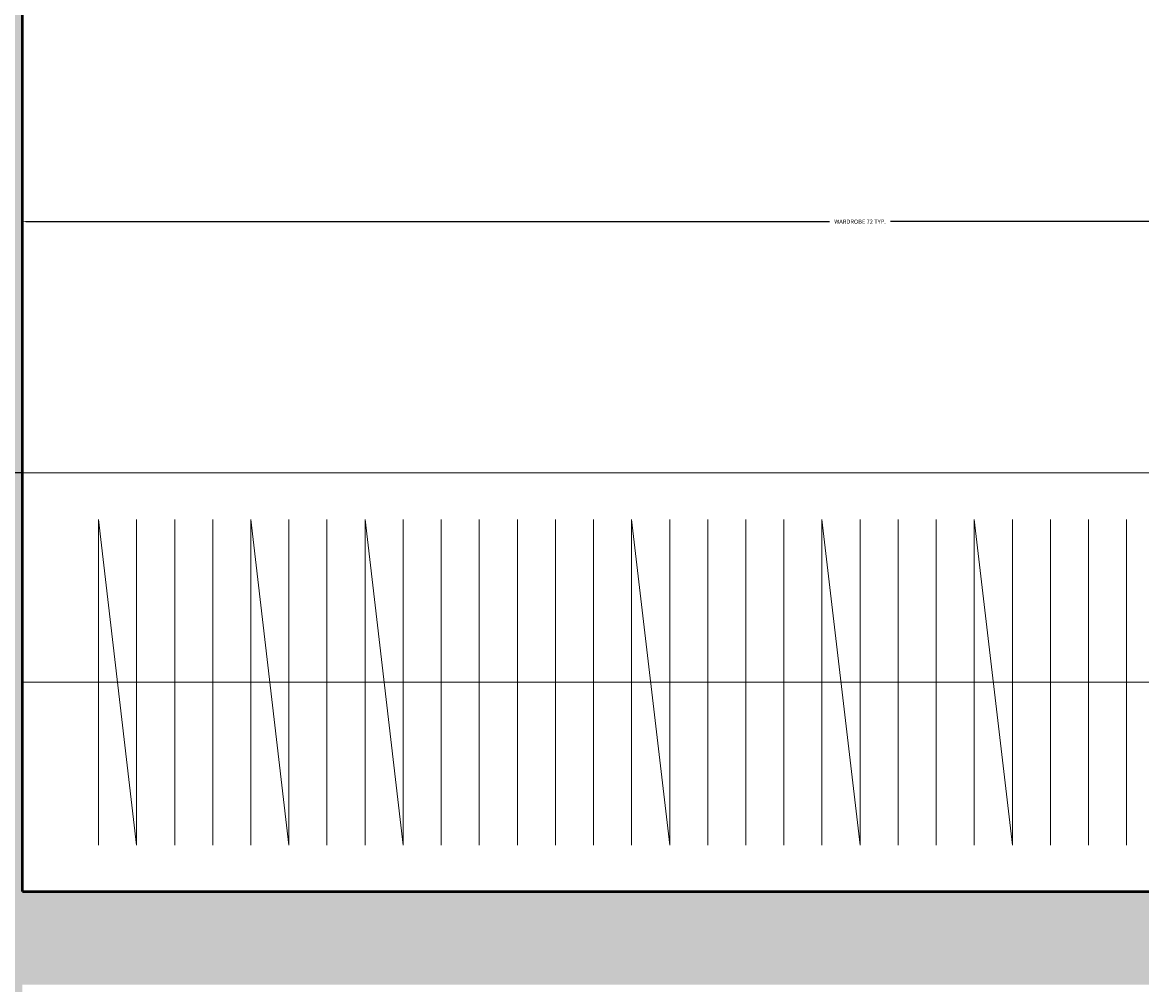
# Model space of a CAD drawing. Units: inches. Extents: x 2307 to 2544, y 2171 to 2540.
# Tile 17 of 52: x 2336 to 2384, y 2388 to 2429. Entities that reach past the tile are written whole.
import ezdxf

# ---------------------------------------------------------------- set-up
doc = ezdxf.new("R2010")
doc.units = ezdxf.units.IN
for name, color, linetype, lineweight in [('A-ANNO-DIMS', 2, 'Continuous', 18), ('A-FLOR-CASE', 9, 'Continuous', 18), ('A-WALL', 7, 'Continuous', 50)]:
    doc.layers.add(name, color=color, linetype=linetype, lineweight=lineweight)
doc.layers.add('A-WALL-PATT', color=18, linetype='Continuous', lineweight=13, true_color=0x000000)
doc.styles.get("Standard").update_dxf_attribs({"font": 'arial.ttf'})
doc.dimstyles.get("Standard").update_dxf_attribs({"dimtxt": 0.18, "dimasz": 0.18, "dimexe": 0.18, "dimexo": 0.0625, "dimgap": 0.09, "dimtad": 0, "dimtih": 1, "dimtoh": 1, "dimdec": 4, "dimzin": 0, "dimdsep": 46, "dimtxsty": 'Standard', "dimcen": 0.09, "dimadec": 0, "dimazin": 0, "dimtfac": 1, "dimtdec": 4, "dimtofl": 0, "dimtmove": 0, "dimatfit": 3, "dimfxl": 1, "dimtolj": 1, "dimtzin": 0, "dimarcsym": 0})

# ---------------------------------------------------------------- blocks, each defined once
blk = doc.blocks.new('WARDROBE-72X18IN')
for p, q in [((0, 72), (0, 0)), ((18, 72), (0, 72)), ((9, 72), (9, 0)), ((18, 0), (18, 72)), ((16, 68.727), (2, 68.727)), ((16, 68.727), (2, 67.09)), ((16, 67.09), (2, 67.09)), ((16, 65.454), (2, 65.454)), ((16, 63.818), (2, 63.818)), ((16, 62.181), (2, 62.181)), ((16, 62.181), (2, 60.545)), ((16, 60.545), (2, 60.545)), ((16, 58.909), (2, 58.909)), ((16, 57.272), (2, 57.272)), ((16, 57.272), (2, 55.636)), ((16, 55.636), (2, 55.636)), ((16, 54), (2, 54)), ((16, 52.363), (2, 52.363)), ((16, 50.727), (2, 50.727)), ((16, 49.09), (2, 49.09)), ((16, 47.454), (2, 47.454)), ((16, 45.818), (2, 45.818)), ((16, 45.818), (2, 44.181)), ((16, 44.181), (2, 44.181)), ((16, 42.545), (2, 42.545)), ((16, 40.909), (2, 40.909)), ((16, 39.272), (2, 39.272)), ((16, 37.636), (2, 37.636)), ((16, 37.636), (2, 36)), ((16, 36), (2, 36)), ((16, 34.363), (2, 34.363)), ((16, 32.727), (2, 32.727)), ((16, 31.09), (2, 31.09)), ((16, 31.09), (2, 29.454)), ((16, 29.454), (2, 29.454)), ((16, 27.818), (2, 27.818)), ((16, 26.181), (2, 26.181)), ((16, 24.545), (2, 24.545)), ((16, 22.909), (2, 22.909)), ((16, 21.272), (2, 21.272)), ((16, 19.636), (2, 19.636)), ((16, 18), (2, 18)), ((16, 18), (2, 16.363)), ((16, 16.363), (2, 16.363)), ((16, 14.727), (2, 14.727)), ((16, 13.09), (2, 13.09)), ((16, 11.454), (2, 11.454)), ((16, 11.454), (2, 9.818)), ((16, 9.818), (2, 9.818)), ((16, 8.181), (2, 8.181)), ((16, 6.545), (2, 6.545)), ((16, 4.909), (2, 4.909)), ((16, 3.272), (2, 3.272)), ((0, 0), (18, 0)), ((18, 0), (0, 0))]:
    blk.add_line(p, q)
blk = doc.blocks.new('*D18')
at = {"layer": 'A-ANNO-DIMS', "color": 0, "lineweight": -2, "transparency": 16777216}
for p, q in [((2335.696, 2409.572), (2335.696, 2420.49)), ((2407.696, 2409.572), (2407.696, 2420.49)), ((2335.876, 2420.31), (2370.389, 2420.31)), ((2407.516, 2420.31), (2373.003, 2420.31))]:
    blk.add_line(p, q, dxfattribs=at)
at = {"layer": 'A-ANNO-DIMS', "color": 0, "transparency": 16777216}
for points in [[(2335.876, 2420.34), (2335.876, 2420.28), (2335.696, 2420.31)], [(2407.516, 2420.34), (2407.516, 2420.28), (2407.696, 2420.31)]]:
    blk.add_solid(points, dxfattribs=at)
at = {"layer": 'Defpoints', "color": 0, "transparency": 16777216}
for p in [(2335.696, 2420.31), (2335.696, 2409.51), (2407.696, 2409.51)]:
    blk.add_point(p, dxfattribs=at)
at = {"layer": 'A-ANNO-DIMS', "color": 0, "transparency": 16777216, "insert": (2371.696, 2420.31), "char_height": 0.18, "attachment_point": 5}
blk.add_mtext('\\A1;WARDROBE 72 TYP.', dxfattribs=at)
blk = doc.blocks.new('*D67')
at = {"layer": 'A-ANNO-DIMS', "color": 0, "lineweight": -2, "transparency": 16777216}
for p, q in [((2339.646, 2432.174), (2307.366, 2432.174)), ((2307.546, 2431.994), (2307.546, 2421.024)), ((2307.546, 2409.69), (2307.546, 2420.66)), ((2335.633, 2409.51), (2307.366, 2409.51))]:
    blk.add_line(p, q, dxfattribs=at)
at = {"layer": 'A-ANNO-DIMS', "color": 0, "transparency": 16777216}
for points in [[(2307.516, 2431.994), (2307.576, 2431.994), (2307.546, 2432.174)], [(2307.516, 2409.69), (2307.576, 2409.69), (2307.546, 2409.51)]]:
    blk.add_solid(points, dxfattribs=at)
at = {"layer": 'Defpoints', "color": 0, "transparency": 16777216}
for p in [(2307.546, 2432.174), (2339.708, 2432.174), (2335.696, 2409.51)]:
    blk.add_point(p, dxfattribs=at)
at = {"layer": 'A-ANNO-DIMS', "color": 0, "transparency": 16777216, "insert": (2307.546, 2420.842), "char_height": 0.18, "attachment_point": 5}
blk.add_mtext('\\A1;22.665', dxfattribs=at)

msp = doc.modelspace()

# ---------------------------------------------------------------- hatches: boundary and pattern name
at = {"layer": 'A-WALL-PATT'}
h = msp.add_hatch(color=256, dxfattribs=at)
h.dxf.hatch_style = 1
h.paths.add_polyline_path([(2367.4028, 2520.5096), (2326.6958, 2520.5096), (2326.6958, 2355.3983), (2335.6958, 2355.3983), (2335.6958, 2387.5096), (2415.6958, 2387.5096), (2415.6958, 2391.5096), (2335.6958, 2391.5096), (2335.6958, 2409.5096), (2335.6958, 2511.5096), (2367.4028, 2511.5096)])

# ---------------------------------------------------------------- linework, layer by layer
at = {"layer": 'A-WALL'}
for q in [(2335.6958, 2511.5096), (2415.6958, 2391.5096)]:
    msp.add_line((2335.6958, 2391.5096), q, dxfattribs=at)

# ---------------------------------------------------------------- block references
at = {"layer": 'A-FLOR-CASE', "rotation": 90.00000000000885}
msp.add_blockref('WARDROBE-72X18IN', (2407.6954, 2391.5097), dxfattribs=at)

# ---------------------------------------------------------------- dimensions: what is measured, and where the dimension line sits
at = {"layer": 'A-ANNO-DIMS'}
dim = msp.add_linear_dim(base=(2307.5458, 2432.1742), p1=(2335.6958, 2409.5096), p2=(2339.7083, 2432.1742), angle=90, dimstyle='Standard', override={"dimdec": 3, "dimlfac": 1, "dimrnd": 0, "dimzin": 0, "dimdsep": 46, "dimlunit": 2}, dxfattribs=at)
dim.commit()
dim.dimension.update_dxf_attribs({"geometry": '*D67', "text_midpoint": (2307.5458, 2420.8419)})
dim = msp.add_linear_dim(base=(2335.6958, 2420.3096), p1=(2407.6958, 2409.5096), p2=(2335.6958, 2409.5096), angle=180, text='WARDROBE <> TYP.', dimstyle='Standard', override={"dimdec": 0, "dimlfac": 1, "dimrnd": 0, "dimzin": 0, "dimdsep": 46, "dimlunit": 2}, dxfattribs=at)
dim.commit()
dim.dimension.update_dxf_attribs({"geometry": '*D18', "text_midpoint": (2371.6958, 2420.3096)})

doc.saveas('drawing.dxf')
